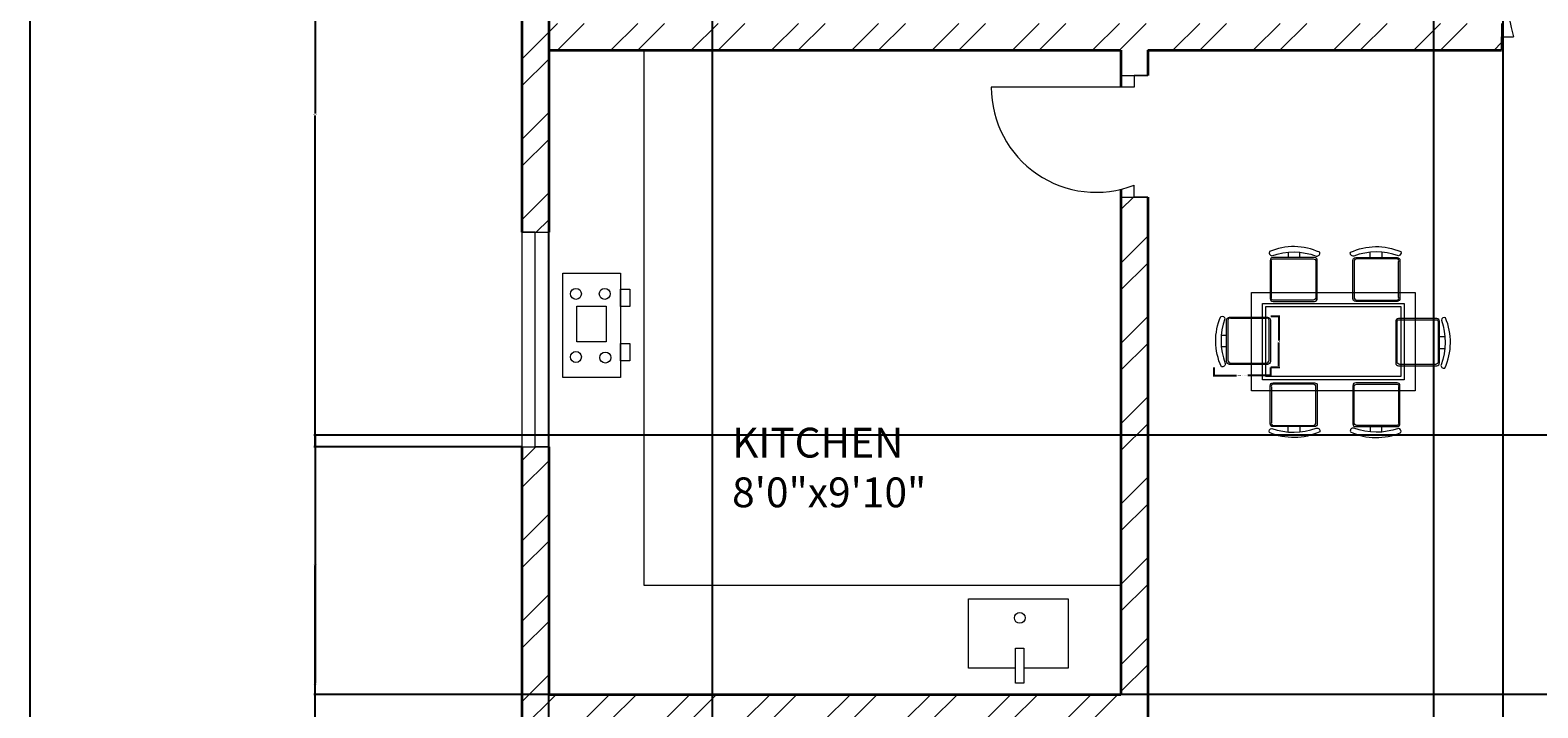
# Model space of a CAD drawing. Units: inches. Extents: x 1965 to 2673, y 1802 to 2669.
# Tile 6 of 16: x 1965 to 2218, y 2154 to 2267. Entities that reach past the tile are written whole.
import ezdxf

# ---------------------------------------------------------------- set-up
doc = ezdxf.new("R2010")
doc.units = ezdxf.units.IN
for name, color, linetype, lineweight in [('A-ANNO-DIMS', 2, 'Continuous', 18), ('A-ANNO-TTLB', 7, 'Continuous', 25), ('A-AREA-IDEN', 7, 'Continuous', 18), ('A-DOOR', 11, 'Continuous', 18), ('A-EQPM', 8, 'Continuous', 18), ('A-FLOR-CASE', 8, 'Continuous', 18), ('A-FLOR-FIXT', 9, 'Continuous', 18), ('A-FURN', 8, 'Continuous', 13), ('A-GLAZ', 181, 'Continuous', 18), ('A-WALL', 7, 'Continuous', 35), ('A-WALL-PATT', 252, 'Continuous', 13)]:
    doc.layers.add(name, color=color, linetype=linetype, lineweight=lineweight)
doc.styles.get("Standard").update_dxf_attribs({"font": 'arial.ttf'})
doc.dimstyles.get("Standard").update_dxf_attribs({"dimtxt": 0.18, "dimasz": 0.18, "dimexe": 0.18, "dimexo": 0.0625, "dimgap": 0.09, "dimtad": 0, "dimtih": 1, "dimtoh": 1, "dimdec": 4, "dimzin": 0, "dimdsep": 46, "dimtxsty": 'Standard', "dimcen": 0.09, "dimadec": 0, "dimazin": 0, "dimtfac": 1, "dimtdec": 4, "dimtofl": 0, "dimtmove": 0, "dimatfit": 3, "dimfxl": 1, "dimtolj": 1, "dimtzin": 0, "dimarcsym": 0})

# ---------------------------------------------------------------- blocks, each defined once
blk = doc.blocks.new('WIN-36IN')
for p, q in [((2.25, 36.01), (0, 36.01)), ((0, 36.01), (4.5, 36.01)), ((0, 36.01), (0, 0.01)), ((2.25, 0.01), (2.25, 36.01)), ((4.5, 36.01), (4.5, 0.01)), ((0, 0.01), (4.5, 0.01)), ((4.5, 0.01), (2.25, 0.01))]:
    blk.add_line(p, q)
blk = doc.blocks.new('TABLE-DINING-RECT')
for points in [[(0, 16.47), (27.44, 16.47), (27.44, 0), (0, 0)], [(0, 16.47), (27.44, 16.47), (27.44, 0), (0, 0)], [(1.83, 14.64), (25.61, 14.64), (25.61, 1.83), (1.83, 1.83)], [(1.83, 14.64), (25.61, 14.64), (25.61, 1.83), (1.83, 1.83)], [(2.38, 14.09), (25.06, 14.09), (25.06, 2.38), (2.38, 2.38)], [(2.38, 14.09), (25.06, 14.09), (25.06, 2.38), (2.38, 2.38)]]:
    blk.add_lwpolyline(points, close=True)
blk = doc.blocks.new('CHAIR-DINING')
for points in [[(1.58, 0.59, -0.578392), (0.96, 0.02, -0.214524), (0.85, 8.46, -0.552014), (1.52, 8.06, 0.175809), (1.58, 0.59)], [(1.58, 0.59, -0.578392), (0.96, 0.02, -0.214524), (0.85, 8.46, -0.552014), (1.52, 8.06, 0.175809), (1.58, 0.59)], [(1.82, 7.85, -0.414214), (2.31, 8.33), (8.69, 8.33, -0.414214), (9.18, 7.85), (9.18, 0.91, -0.414214), (8.69, 0.42), (2.31, 0.42, -0.414214), (1.82, 0.91), (1.82, 7.85)], [(1.82, 7.85, -0.414214), (2.31, 8.33), (8.69, 8.33, -0.414214), (9.18, 7.85), (9.18, 0.91, -0.414214), (8.69, 0.42), (2.31, 0.42, -0.414214), (1.82, 0.91), (1.82, 7.85)], [(1.82, 3.34), (0.95, 3.34, 0.064759)], [(1.82, 3.34), (0.95, 3.34, 0.064759)]]:
    blk.add_lwpolyline(points, format="xyb")
blk.add_lwpolyline([(2.04, 7.84), (2.04, 1.12, 0.414214), (2.53, 0.64), (8.47, 0.64, 0.414214), (8.96, 1.12), (8.96, 7.84, 0.512069), (8.47, 8.11), (2.53, 8.11, 0.512069)], format="xyb", close=True)
blk.add_lwpolyline([(2.04, 7.84), (2.04, 1.12, 0.414214), (2.53, 0.64), (8.47, 0.64, 0.414214), (8.96, 1.12), (8.96, 7.84, 0.512069), (8.47, 8.11), (2.53, 8.11, 0.512069)], format="xyb", close=True)
blk.add_lwpolyline([(0.93, 5.29), (1.82, 5.29)])
blk.add_lwpolyline([(0.93, 5.29), (1.82, 5.29)])
blk = doc.blocks.new('*D21')
at = {"layer": 'A-ANNO-DIMS', "color": 0, "lineweight": -2, "transparency": 16777216}
for p, q in [((2163.18, 2210.92), (2163.18, 2209.37)), ((2163.36, 2209.55), (2166.98, 2209.55)), ((2172.51, 2209.55), (2168.89, 2209.55)), ((2172.69, 2210.92), (2172.69, 2209.37))]:
    blk.add_line(p, q, dxfattribs=at)
at = {"layer": 'A-ANNO-DIMS', "color": 0, "transparency": 16777216}
for points in [[(2163.36, 2209.58), (2163.36, 2209.52), (2163.18, 2209.55)], [(2172.51, 2209.58), (2172.51, 2209.52), (2172.69, 2209.55)]]:
    blk.add_solid(points, dxfattribs=at)
at = {"layer": 'Defpoints', "color": 0, "transparency": 16777216}
for p in [(2163.18, 2210.98), (2172.69, 2210.98), (2172.69, 2209.55)]:
    blk.add_point(p, dxfattribs=at)
at = {"layer": 'A-ANNO-DIMS', "color": 0, "transparency": 16777216, "insert": (2167.94, 2209.55), "char_height": 0.18, "attachment_point": 5}
blk.add_mtext('\\A1;CHAIR 10 TYP.', dxfattribs=at)
blk = doc.blocks.new('*D22')
at = {"layer": 'A-ANNO-DIMS', "color": 0, "lineweight": -2, "transparency": 16777216}
for p, q in [((2172.75, 2219.54), (2174.29, 2219.54)), ((2174.11, 2219.36), (2174.11, 2215.44)), ((2174.11, 2211.16), (2174.11, 2215.08)), ((2172.75, 2210.98), (2174.29, 2210.98))]:
    blk.add_line(p, q, dxfattribs=at)
at = {"layer": 'A-ANNO-DIMS', "color": 0, "transparency": 16777216}
for points in [[(2174.08, 2219.36), (2174.14, 2219.36), (2174.11, 2219.54)], [(2174.08, 2211.16), (2174.14, 2211.16), (2174.11, 2210.98)]]:
    blk.add_solid(points, dxfattribs=at)
at = {"layer": 'Defpoints', "color": 0, "transparency": 16777216}
for p in [(2172.69, 2219.54), (2174.11, 2219.54), (2172.69, 2210.98)]:
    blk.add_point(p, dxfattribs=at)
at = {"layer": 'A-ANNO-DIMS', "color": 0, "transparency": 16777216, "insert": (2174.11, 2215.26), "char_height": 0.18, "attachment_point": 5}
blk.add_mtext('\\A1;9 TYP.', dxfattribs=at)
blk = doc.blocks.new('*D35')
at = {"layer": 'A-ANNO-DIMS', "color": 0, "lineweight": -2, "transparency": 16777216}
for p, q in [((2047.03, 2197.58), (2012.19, 2197.58)), ((2012.37, 2197.4), (2012.37, 2157.95)), ((2012.37, 2118.13), (2012.37, 2157.59)), ((2047.03, 2117.95), (2012.19, 2117.95))]:
    blk.add_line(p, q, dxfattribs=at)
at = {"layer": 'A-ANNO-DIMS', "color": 0, "transparency": 16777216}
for points in [[(2012.34, 2197.4), (2012.4, 2197.4), (2012.37, 2197.58)], [(2012.34, 2118.13), (2012.4, 2118.13), (2012.37, 2117.95)]]:
    blk.add_solid(points, dxfattribs=at)
at = {"layer": 'Defpoints', "color": 0, "transparency": 16777216}
for p in [(2012.37, 2197.58), (2047.09, 2197.58), (2047.09, 2117.95)]:
    blk.add_point(p, dxfattribs=at)
at = {"layer": 'A-ANNO-DIMS', "color": 0, "transparency": 16777216, "insert": (2012.37, 2157.77), "char_height": 0.18, "attachment_point": 5}
blk.add_mtext('\\A1;79.63', dxfattribs=at)
blk = doc.blocks.new('*D36')
at = {"layer": 'A-ANNO-DIMS', "color": 0, "lineweight": -2, "transparency": 16777216}
for p, q in [((2047.03, 2309.07), (2012.19, 2309.07)), ((2012.37, 2308.89), (2012.37, 2253.51)), ((2012.37, 2197.76), (2012.37, 2253.14)), ((2047.03, 2197.58), (2012.19, 2197.58))]:
    blk.add_line(p, q, dxfattribs=at)
at = {"layer": 'A-ANNO-DIMS', "color": 0, "transparency": 16777216}
for points in [[(2012.34, 2308.89), (2012.4, 2308.89), (2012.37, 2309.07)], [(2012.34, 2197.76), (2012.4, 2197.76), (2012.37, 2197.58)]]:
    blk.add_solid(points, dxfattribs=at)
at = {"layer": 'Defpoints', "color": 0, "transparency": 16777216}
for p in [(2012.37, 2309.07), (2047.09, 2309.07), (2047.09, 2197.58)]:
    blk.add_point(p, dxfattribs=at)
at = {"layer": 'A-ANNO-DIMS', "color": 0, "transparency": 16777216, "insert": (2012.37, 2253.33), "char_height": 0.18, "attachment_point": 5}
blk.add_mtext('\\A1;111.49', dxfattribs=at)
blk = doc.blocks.new('*D39')
at = {"layer": 'A-ANNO-DIMS', "color": 0, "lineweight": -2, "transparency": 16777216}
for p, q in [((2051.59, 1936.15), (2051.59, 2600.5)), ((2051.77, 2600.32), (2064.93, 2600.32)), ((2078.87, 2600.32), (2065.72, 2600.32)), ((2079.05, 1936.15), (2079.05, 2600.5))]:
    blk.add_line(p, q, dxfattribs=at)
at = {"layer": 'A-ANNO-DIMS', "color": 0, "transparency": 16777216}
for points in [[(2051.77, 2600.35), (2051.77, 2600.29), (2051.59, 2600.32)], [(2078.87, 2600.35), (2078.87, 2600.29), (2079.05, 2600.32)]]:
    blk.add_solid(points, dxfattribs=at)
at = {"layer": 'Defpoints', "color": 0, "transparency": 16777216}
for p in [(2079.05, 2600.32), (2051.59, 1936.09), (2079.05, 1936.09)]:
    blk.add_point(p, dxfattribs=at)
at = {"layer": 'A-ANNO-DIMS', "color": 0, "transparency": 16777216, "insert": (2065.32, 2600.32), "char_height": 0.18, "attachment_point": 5}
blk.add_mtext('\\A1;27.46', dxfattribs=at)
blk = doc.blocks.new('*D40')
at = {"layer": 'A-ANNO-DIMS', "color": 0, "lineweight": -2, "transparency": 16777216}
for p, q in [((2200.09, 1936.15), (2200.09, 2600.5)), ((2200.27, 2600.32), (2205.48, 2600.32)), ((2211.59, 2600.32), (2206.38, 2600.32)), ((2211.77, 1936.15), (2211.77, 2600.5))]:
    blk.add_line(p, q, dxfattribs=at)
at = {"layer": 'A-ANNO-DIMS', "color": 0, "transparency": 16777216}
for points in [[(2200.27, 2600.35), (2200.27, 2600.29), (2200.09, 2600.32)], [(2211.59, 2600.35), (2211.59, 2600.29), (2211.77, 2600.32)]]:
    blk.add_solid(points, dxfattribs=at)
at = {"layer": 'Defpoints', "color": 0, "transparency": 16777216}
for p in [(2211.77, 2600.32), (2200.09, 1936.09), (2211.77, 1936.09)]:
    blk.add_point(p, dxfattribs=at)
at = {"layer": 'A-ANNO-DIMS', "color": 0, "transparency": 16777216, "insert": (2205.93, 2600.32), "char_height": 0.18, "attachment_point": 5}
blk.add_mtext('\\A1;11.674', dxfattribs=at)
blk = doc.blocks.new('*D47')
at = {"layer": 'A-ANNO-DIMS', "color": 0, "lineweight": -2, "transparency": 16777216}
for p, q in [((2573.53, 2199.58), (2012.19, 2199.58)), ((2012.37, 2199.4), (2012.37, 2178.02)), ((2012.37, 2156.27), (2012.37, 2177.65)), ((2573.53, 2156.09), (2012.19, 2156.09))]:
    blk.add_line(p, q, dxfattribs=at)
at = {"layer": 'A-ANNO-DIMS', "color": 0, "transparency": 16777216}
for points in [[(2012.34, 2199.4), (2012.4, 2199.4), (2012.37, 2199.58)], [(2012.34, 2156.27), (2012.4, 2156.27), (2012.37, 2156.09)]]:
    blk.add_solid(points, dxfattribs=at)
at = {"layer": 'Defpoints', "color": 0, "transparency": 16777216}
for p in [(2012.37, 2199.58), (2573.59, 2199.58), (2573.59, 2156.09)]:
    blk.add_point(p, dxfattribs=at)
at = {"layer": 'A-ANNO-DIMS', "color": 0, "transparency": 16777216, "insert": (2012.37, 2177.83), "char_height": 0.18, "attachment_point": 5}
blk.add_mtext('\\A1;43.48', dxfattribs=at)

msp = doc.modelspace()

# ---------------------------------------------------------------- hatches: boundary and pattern name
at = {"layer": 'A-WALL-PATT'}
h = msp.add_hatch(dxfattribs=at)
h.set_pattern_fill('ANSI32', color=256)
h.paths.add_polyline_path([(2051.5927, 2561.0914), (2076.7559, 2561.0914), (2076.7559, 2563.3414), (2076.7559, 2565.5914), (2047.0927, 2565.5914), (2047.0927, 2518.3824), (2051.5927, 2518.3824)])
h.paths.add_polyline_path([(2051.5927, 2458.3824), (2049.3427, 2458.3824), (2047.0927, 2458.3824), (2047.0927, 2412.5914), (2248.0927, 2412.5914), (2248.0927, 2268.5914), (2252.5927, 2268.5914), (2252.5927, 2412.5914), (2252.5927, 2421.0404), (2250.3427, 2421.0404), (2248.0927, 2421.0404), (2248.0927, 2417.0914), (2051.5927, 2417.0914)])
h.paths.add_polyline_path([(2211.4933, 2268.5914), (2104.0927, 2268.5914), (2104.0927, 2272.4654), (2101.8427, 2272.4654), (2099.5927, 2272.4654), (2099.5927, 2268.5914), (2051.5927, 2268.5914), (2051.5927, 2264.0914), (2147.5927, 2264.0914), (2147.5927, 2259.8893), (2152.0927, 2259.8893), (2152.0927, 2264.0914), (2211.4933, 2264.0914), (2211.4933, 2266.3414)])
h.paths.add_polyline_path([(2104.0927, 2376.0914), (2099.5927, 2376.0914), (2047.0927, 2376.0914), (2047.0927, 2333.0682), (2051.5927, 2333.0682), (2051.5927, 2371.5914), (2099.5927, 2371.5914), (2099.5927, 2293.6123), (2104.0927, 2293.6123)], flags=17)
h.paths.add_polyline_path([(2051.5927, 2309.0682), (2047.0927, 2309.0682), (2047.0927, 2233.5821), (2051.5927, 2233.5821)])
h.paths.add_polyline_path([(2104.0927, 2412.5914), (2099.5927, 2412.5914), (2099.5927, 2376.0914), (2104.0927, 2376.0914)], flags=17)
h.paths.add_polyline_path([(2290.1254, 2268.5914), (2242.4924, 2268.5914), (2242.4924, 2264.0914), (2290.1254, 2264.0914), (2290.1254, 2266.3414)])
h.paths.add_polyline_path([(2284.653, 2264.0914), (2280.153, 2264.0914), (2280.153, 2161.6826), (2284.653, 2161.6826)])
h.paths.add_polyline_path([(2578.0927, 2329.4656), (2573.5927, 2329.4656), (2573.5927, 2268.5914), (2525.5927, 2268.5914), (2525.5927, 2271.9222), (2523.3427, 2271.9222), (2521.0927, 2271.9222), (2521.0927, 2268.5914), (2324.2835, 2268.5914), (2324.2835, 2264.0914), (2329.0927, 2264.0914), (2329.0927, 2259.4977), (2333.5927, 2259.4977), (2333.5927, 2264.0914), (2473.0927, 2264.0914), (2473.0927, 2259.9371), (2477.5927, 2259.9371), (2477.5927, 2264.0914), (2573.5927, 2264.0914), (2573.5927, 2235.5751), (2578.0927, 2235.5751)])
h.paths.add_polyline_path([(2377.0927, 2412.5914), (2578.0927, 2412.5914), (2578.0927, 2444.2286), (2575.8427, 2444.2286), (2573.5927, 2444.2286), (2573.5927, 2417.0914), (2429.5927, 2417.0914), (2377.0927, 2417.0914), (2377.0927, 2421.7443), (2372.5927, 2421.7443), (2372.5927, 2268.5914), (2377.0927, 2268.5914)])
h.paths.add_polyline_path([(2525.5927, 2371.5914), (2573.5927, 2371.5914), (2573.5927, 2353.4656), (2578.0927, 2353.4656), (2578.0927, 2376.0914), (2525.5927, 2376.0914), (2521.0927, 2376.0914), (2521.0927, 2290.6472), (2525.5927, 2290.6472)], flags=17)
h.paths.add_polyline_path([(2477.5927, 2236.4106), (2475.3427, 2236.4106), (2473.0927, 2236.4106), (2473.0927, 2084.5914), (2465.3309, 2084.5914), (2465.3309, 2080.0914), (2481.6764, 2080.0914), (2481.6764, 2082.3414), (2481.6764, 2084.5914), (2477.5927, 2084.5914), (2477.5927, 2151.5914), (2573.5927, 2151.5914), (2573.5927, 2130.2907), (2578.0927, 2130.2907), (2578.0927, 2199.5751), (2575.8427, 2199.5751), (2573.5927, 2199.5751), (2573.5927, 2156.0914), (2477.5927, 2156.0914)])
h.paths.add_polyline_path([(2573.5927, 2084.5914), (2505.5513, 2084.5914), (2505.5513, 2080.0914), (2573.5927, 2080.0914)], flags=17)
h.paths.add_polyline_path([(2578.0927, 2106.2907), (2575.8427, 2106.2907), (2573.5927, 2106.2907), (2573.5927, 2050.8986), (2578.0927, 2050.8986)])
h.paths.add_polyline_path([(2578.0927, 1990.8986), (2575.8427, 1990.8986), (2573.5927, 1990.8986), (2573.5927, 1936.0914), (2522.132, 1936.0914), (2522.132, 1931.5914), (2578.0927, 1931.5914)])
h.paths.add_polyline_path([(2462.132, 1936.0914), (2429.5927, 1936.0914), (2429.5927, 2080.0914), (2432.623, 2080.0914), (2432.623, 2082.3414), (2432.623, 2084.5914), (2429.5927, 2084.5914), (2429.5927, 2120.5914), (2333.5927, 2120.5914), (2333.5927, 2229.3125), (2331.3427, 2229.3125), (2329.0927, 2229.3125), (2329.0927, 2116.0914), (2425.0927, 2116.0914), (2425.0927, 1936.0914), (2346.4058, 1936.0914), (2346.4058, 1931.5914), (2462.132, 1931.5914), (2462.132, 1933.8414)])
h.paths.add_polyline_path([(2211.767, 1933.8414), (2211.767, 1936.0914), (2200.0927, 1936.0914), (2200.0927, 2080.0914), (2200.0927, 2116.0914), (2284.653, 2116.0914), (2284.653, 2130.591), (2282.403, 2130.591), (2280.153, 2130.591), (2280.153, 2120.5914), (2200.0927, 2120.5914), (2195.5927, 2120.5914), (2195.5927, 2080.0914), (2195.5927, 1936.0914), (2139.0533, 1936.0914), (2139.0533, 1931.5914), (2211.767, 1931.5914)])
h.paths.add_polyline_path([(2282.2502, 1933.8414), (2282.2502, 1936.0914), (2259.767, 1936.0914), (2259.767, 1931.5914), (2282.2502, 1931.5914)], flags=17)
h.paths.add_polyline_path([(2051.5927, 1987.096), (2049.3427, 1987.096), (2047.0927, 1987.096), (2047.0927, 1931.5914), (2079.0533, 1931.5914), (2079.0533, 1933.8414), (2079.0533, 1936.0914), (2051.5927, 1936.0914)])
h.paths.add_polyline_path([(2051.5927, 2197.5821), (2049.3427, 2197.5821), (2047.0927, 2197.5821), (2047.0927, 2141.952), (2051.5927, 2141.952), (2051.5927, 2151.5914), (2147.5927, 2151.5914), (2147.5927, 2084.5914), (2144.3652, 2084.5914), (2144.3652, 2080.0914), (2155.9662, 2080.0914), (2155.9662, 2082.3414), (2155.9662, 2084.5914), (2152.0927, 2084.5914), (2152.0927, 2239.4921), (2149.8427, 2239.4921), (2147.5927, 2239.4921), (2147.5927, 2156.0914), (2051.5927, 2156.0914)])
h.paths.add_polyline_path([(2051.5927, 2080.0914), (2123.8575, 2080.0914), (2123.8575, 2082.3414), (2123.8575, 2084.5914), (2051.5927, 2084.5914), (2051.5927, 2117.952), (2047.0927, 2117.952), (2047.0927, 2047.096), (2051.5927, 2047.096)])
h = msp.add_hatch(dxfattribs=at)
h.set_pattern_fill('ANSI32', color=256)
h.paths.add_polyline_path([(2210.2316, 2563.3414), (2210.2316, 2565.5914), (2136.7559, 2565.5914), (2136.7559, 2561.0914), (2195.5927, 2561.0914), (2195.5927, 2485.8604), (2200.0927, 2485.8604), (2200.0927, 2561.0914), (2210.2316, 2561.0914)])
h.paths.add_polyline_path([(2285.9734, 2565.5914), (2234.2316, 2565.5914), (2234.2316, 2561.0914), (2248.0927, 2561.0914), (2248.0927, 2462.0914), (2200.0927, 2462.0914), (2200.0927, 2465.2357), (2197.8427, 2465.2357), (2195.5927, 2465.2357), (2195.5927, 2457.5914), (2248.0927, 2457.5914), (2248.0927, 2452.628), (2252.5927, 2452.628), (2252.5927, 2457.5914), (2257.5156, 2457.5914), (2257.5156, 2459.8414), (2257.5156, 2462.0914), (2252.5927, 2462.0914), (2252.5927, 2561.0914), (2285.9734, 2561.0914)])
h.paths.add_polyline_path([(2213.1374, 1872.8885), (2461.061, 1872.8885), (2461.061, 1909.9813), (2213.1374, 1909.9813)], flags=9)
h.paths.add_polyline_path([(2328.4056, 1942.3944), (2340.6089, 1942.3944), (2340.6089, 1952.6979), (2328.4056, 1952.6979)], flags=9)
h.paths.add_polyline_path([(2353.5759, 2030.9808), (2376.6455, 2030.9808), (2376.6455, 2041.2844), (2353.5759, 2041.2844)], flags=9)
h.paths.add_polyline_path([(2289.989, 2074.1041), (2326.916, 2074.1041), (2326.916, 2092.7615), (2289.989, 2092.7615)], flags=9)
h.paths.add_polyline_path([(2497.9, 2052.8638), (2548.3741, 2052.8638), (2548.3741, 2071.5212), (2497.9, 2071.5212)], flags=9)
h.paths.add_polyline_path([(2486.59, 2116.4883), (2515.7475, 2116.4883), (2515.7475, 2135.1456), (2486.59, 2135.1456)], flags=9)
h.paths.add_polyline_path([(2497.3007, 2181.2877), (2530.459, 2181.2877), (2530.459, 2199.945), (2497.3007, 2199.945)], flags=9)
h.paths.add_polyline_path([(2288.237, 2190.3228), (2324.1238, 2190.3228), (2324.1238, 2208.9802), (2288.237, 2208.9802)], flags=9)
h.paths.add_polyline_path([(2350.806, 2127.8307), (2387.733, 2127.8307), (2387.733, 2146.488), (2350.806, 2146.488)], flags=9)
h.paths.add_polyline_path([(2530.3237, 2315.2679), (2559.5563, 2315.2679), (2559.5563, 2333.9252), (2530.3237, 2333.9252)], flags=9)
h.paths.add_polyline_path([(2418.419, 2383.4707), (2468.2894, 2383.4707), (2468.2894, 2402.1281), (2418.419, 2402.1281)], flags=9)
h.paths.add_polyline_path([(2327.4503, 2399.0281), (2364.3773, 2399.0281), (2364.3773, 2417.6854), (2327.4503, 2417.6854)], flags=9)
h.paths.add_polyline_path([(2147.9722, 2271.4601), (2197.8426, 2271.4601), (2197.8426, 2290.1174), (2147.9722, 2290.1174)], flags=9)
h.paths.add_polyline_path([(2474.3875, 2421.594), (2524.8616, 2421.594), (2524.8616, 2440.2514), (2474.3875, 2440.2514)], flags=9)
h.paths.add_polyline_path([(2063.9863, 2052.9059), (2114.4604, 2052.9059), (2114.4604, 2071.5632), (2063.9863, 2071.5632)], flags=9)
h.paths.add_polyline_path([(2200.3335, 2133.7067), (2237.2605, 2133.7067), (2237.2605, 2152.364), (2200.3335, 2152.364)], flags=9)
h.paths.add_polyline_path([(2080.5973, 2184.636), (2113.8681, 2184.636), (2113.8681, 2203.2933), (2080.5973, 2203.2933)], flags=9)
h.paths.add_polyline_path([(2102.4918, 2116.4497), (2131.6494, 2116.4497), (2131.6494, 2135.107), (2102.4918, 2135.107)], flags=9)
h.paths.add_polyline_path([(2056.2753, 2308.5576), (2085.5079, 2308.5576), (2085.5079, 2327.2149), (2056.2753, 2327.2149)], flags=9)
h.paths.add_polyline_path([(2385.619, 2500.9729), (2414.8516, 2500.9729), (2414.8516, 2519.6303), (2385.619, 2519.6303)], flags=9)
h.paths.add_polyline_path([(2286.6643, 2508.6826), (2320.0715, 2508.6826), (2320.0715, 2527.34), (2286.6643, 2527.34)], flags=9)
h.paths.add_polyline_path([(2206.5604, 2500.7243), (2235.793, 2500.7243), (2235.793, 2519.3817), (2206.5604, 2519.3817)], flags=25)
h.paths.add_polyline_path([(2062.6644, 2424.4027), (2112.5348, 2424.4027), (2112.5348, 2443.0601), (2062.6644, 2443.0601)], flags=9)
h = msp.add_hatch(dxfattribs=at)
h.set_pattern_fill('ANSI32', color=256)
h.paths.add_polyline_path([(2429.5927, 2468.6101), (2427.3427, 2468.6101), (2425.0927, 2468.6101), (2425.0927, 2462.0914), (2377.0927, 2462.0914), (2377.0927, 2561.0914), (2390.4173, 2561.0914), (2390.4173, 2565.5914), (2321.9734, 2565.5914), (2321.9734, 2561.0914), (2372.5927, 2561.0914), (2372.5927, 2462.0914), (2281.6605, 2462.0914), (2281.6605, 2457.5914), (2372.5927, 2457.5914), (2372.5927, 2451.3316), (2377.0927, 2451.3316), (2377.0927, 2457.5914), (2429.5927, 2457.5914)])
h.paths.add_polyline_path([(2480.8929, 2565.5914), (2414.4173, 2565.5914), (2414.4173, 2561.0914), (2425.0927, 2561.0914), (2425.0927, 2489.9153), (2429.5927, 2489.9153), (2429.5927, 2561.0914), (2480.8929, 2561.0914), (2480.8929, 2563.3414)])
h.paths.add_polyline_path([(2213.1374, 1872.8885), (2461.061, 1872.8885), (2461.061, 1909.9813), (2213.1374, 1909.9813)], flags=9)
h.paths.add_polyline_path([(2328.4056, 1942.3944), (2340.6089, 1942.3944), (2340.6089, 1952.6979), (2328.4056, 1952.6979)], flags=9)
h.paths.add_polyline_path([(2353.5759, 2030.9808), (2376.6455, 2030.9808), (2376.6455, 2041.2844), (2353.5759, 2041.2844)], flags=9)
h.paths.add_polyline_path([(2289.989, 2074.1041), (2326.916, 2074.1041), (2326.916, 2092.7615), (2289.989, 2092.7615)], flags=9)
h.paths.add_polyline_path([(2497.9, 2052.8638), (2548.3741, 2052.8638), (2548.3741, 2071.5212), (2497.9, 2071.5212)], flags=9)
h.paths.add_polyline_path([(2486.59, 2116.4883), (2515.7475, 2116.4883), (2515.7475, 2135.1456), (2486.59, 2135.1456)], flags=9)
h.paths.add_polyline_path([(2497.3007, 2181.2877), (2530.459, 2181.2877), (2530.459, 2199.945), (2497.3007, 2199.945)], flags=9)
h.paths.add_polyline_path([(2288.237, 2190.3228), (2324.1238, 2190.3228), (2324.1238, 2208.9802), (2288.237, 2208.9802)], flags=9)
h.paths.add_polyline_path([(2350.806, 2127.8307), (2387.733, 2127.8307), (2387.733, 2146.488), (2350.806, 2146.488)], flags=9)
h.paths.add_polyline_path([(2530.3237, 2315.2679), (2559.5563, 2315.2679), (2559.5563, 2333.9252), (2530.3237, 2333.9252)], flags=9)
h.paths.add_polyline_path([(2418.419, 2383.4707), (2468.2894, 2383.4707), (2468.2894, 2402.1281), (2418.419, 2402.1281)], flags=9)
h.paths.add_polyline_path([(2327.4503, 2399.0281), (2364.3773, 2399.0281), (2364.3773, 2417.6854), (2327.4503, 2417.6854)], flags=9)
h.paths.add_polyline_path([(2147.9722, 2271.4601), (2197.8426, 2271.4601), (2197.8426, 2290.1174), (2147.9722, 2290.1174)], flags=9)
h.paths.add_polyline_path([(2474.3875, 2421.594), (2524.8616, 2421.594), (2524.8616, 2440.2514), (2474.3875, 2440.2514)], flags=9)
h.paths.add_polyline_path([(2063.9863, 2052.9059), (2114.4604, 2052.9059), (2114.4604, 2071.5632), (2063.9863, 2071.5632)], flags=9)
h.paths.add_polyline_path([(2200.3335, 2133.7067), (2237.2605, 2133.7067), (2237.2605, 2152.364), (2200.3335, 2152.364)], flags=9)
h.paths.add_polyline_path([(2080.5973, 2184.636), (2113.8681, 2184.636), (2113.8681, 2203.2933), (2080.5973, 2203.2933)], flags=9)
h.paths.add_polyline_path([(2102.4918, 2116.4497), (2131.6494, 2116.4497), (2131.6494, 2135.107), (2102.4918, 2135.107)], flags=9)
h.paths.add_polyline_path([(2056.2753, 2308.5576), (2085.5079, 2308.5576), (2085.5079, 2327.2149), (2056.2753, 2327.2149)], flags=9)
h.paths.add_polyline_path([(2385.619, 2500.9729), (2414.8516, 2500.9729), (2414.8516, 2519.6303), (2385.619, 2519.6303)], flags=25)
h.paths.add_polyline_path([(2286.6643, 2508.6826), (2320.0715, 2508.6826), (2320.0715, 2527.34), (2286.6643, 2527.34)], flags=25)
h.paths.add_polyline_path([(2206.5604, 2500.7243), (2235.793, 2500.7243), (2235.793, 2519.3817), (2206.5604, 2519.3817)], flags=9)
h.paths.add_polyline_path([(2062.6644, 2424.4027), (2112.5348, 2424.4027), (2112.5348, 2443.0601), (2062.6644, 2443.0601)], flags=9)

# ---------------------------------------------------------------- linework, layer by layer
at = {"layer": 'A-ANNO-TTLB'}
msp.add_lwpolyline([(1964.5703, 2669.282), (2673.2605, 2669.282), (2673.2605, 1802.0221), (1964.5703, 1802.0221)], close=True, dxfattribs=at)
at = {"layer": 'A-DOOR'}
for p, q in [((2211.4933, 2268.5914), (2211.4933, 2264.0914)), ((2211.4933, 2264.0914), (2211.4933, 2266.3414)), ((2211.4933, 2266.3414), (2211.4933, 2266.3414)), ((2211.4933, 2266.3414), (2213.4933, 2266.3414)), ((2147.5927, 2259.8893), (2152.0927, 2259.8893)), ((2152.0927, 2259.8893), (2149.8427, 2259.8893)), ((2149.8427, 2259.8893), (2149.8427, 2257.8893)), ((2149.8427, 2257.8893), (2125.8427, 2257.8893)), ((2147.5927, 2239.4921), (2152.0927, 2239.4921)), ((2149.8427, 2239.4921), (2149.8427, 2241.4921)), ((2152.0927, 2239.4921), (2149.8427, 2239.4921))]:
    msp.add_line(p, q, dxfattribs=at)
for centre, radius, start, end in [((2240.4924, 2274.217), 28.1243, 90, 196.261997), ((2143.4441, 2257.8893), 17.6014, 180, 291.317095)]:
    msp.add_arc(centre, radius, start, end, dxfattribs=at)
at = {"layer": 'A-EQPM'}
for points in [[(2053.9419, 2226.7496), (2063.6145, 2226.7496), (2063.6145, 2209.2028), (2053.9419, 2209.2028)], [(2063.6145, 2224.0351), (2065.1828, 2224.0351), (2065.1828, 2221.155), (2063.6145, 2221.155)], [(2056.2917, 2221.2066), (2061.2334, 2221.2066), (2061.2334, 2215.1825), (2056.2917, 2215.1825)], [(2063.6145, 2214.9304), (2065.1828, 2214.9304), (2065.1828, 2212.0503), (2063.6145, 2212.0503)]]:
    msp.add_lwpolyline(points, close=True, dxfattribs=at)
for centre in [(2056.151, 2223.2548), (2060.9924, 2223.2548), (2056.151, 2212.6724), (2061.0928, 2212.572)]:
    msp.add_circle(centre, 0.9237, dxfattribs=at)
at = {"layer": 'A-FLOR-CASE'}
for p, q in [((2067.5569, 2264.0914), (2067.5569, 2174.4181)), ((2067.5569, 2174.4181), (2147.5927, 2174.4181))]:
    msp.add_line(p, q, dxfattribs=at)
at = {"layer": 'A-FLOR-FIXT'}
msp.add_lwpolyline([(2129.9348, 2160.4719), (2122.0193, 2160.4719), (2122.0193, 2172.096), (2138.7623, 2172.096), (2138.7623, 2160.4719), (2131.3354, 2160.4719)], dxfattribs=at)
msp.add_lwpolyline([(2129.9348, 2163.8257), (2131.3354, 2163.8257), (2131.3354, 2157.9973), (2129.9348, 2157.9973)], close=True, dxfattribs=at)
msp.add_circle((2130.6351, 2168.9245), 0.9076, dxfattribs=at)
at = {"layer": 'A-FURN'}
for points in [[(2172.9118, 2229.6509, -0.17580919), (2180.3872, 2229.5943, 0.57839206), (2180.9535, 2230.217, 0.21452438), (2172.5153, 2230.3302, 0.55201397), (2172.9118, 2229.6509, -0.06507904)], [(2172.9118, 2229.6506, -0.17580919), (2180.3872, 2229.594, 0.57839206), (2180.9535, 2230.2167, 0.21452438), (2172.5154, 2230.3299, 0.55201397), (2172.9118, 2229.6506, -0.06507904)], [(2180.0701, 2229.3508), (2173.1301, 2229.3508, 0.41421356), (2172.6446, 2228.8653), (2172.6446, 2222.4842, 0.41421356), (2173.1301, 2221.9987), (2180.0701, 2221.9987, 0.41421356), (2180.5556, 2222.4842), (2180.5556, 2228.8653, 0.41421356), (2180.0701, 2229.3508)], [(2180.0701, 2229.3506), (2173.1301, 2229.3506, 0.41421356), (2172.6446, 2228.865), (2172.6446, 2222.4839, 0.41421356), (2173.1301, 2221.9984), (2180.0701, 2221.9984, 0.41421356), (2180.5556, 2222.4839), (2180.5556, 2228.865, 0.41421356), (2180.0701, 2229.3506)], [(2177.6324, 2229.3508), (2177.6324, 2230.2285, -0.06475861)], [(2177.6324, 2229.3506), (2177.6324, 2230.2282, -0.06475861)], [(2186.6806, 2229.5943, -0.57839206), (2186.1142, 2230.217, -0.21452438), (2194.5524, 2230.3302, -0.55201397), (2194.156, 2229.6509, 0.1758092), (2186.6806, 2229.5943)], [(2186.6806, 2229.594, -0.57839206), (2186.1143, 2230.2167, -0.21452438), (2194.5524, 2230.3299, -0.55201397), (2194.156, 2229.6506, 0.1758092), (2186.6806, 2229.594)], [(2193.9377, 2229.3508, -0.41421356), (2194.4232, 2228.8653), (2194.4232, 2222.4842, -0.41421356), (2193.9377, 2221.9987), (2186.9977, 2221.9987, -0.41421356), (2186.5122, 2222.4842), (2186.5122, 2228.8653, -0.41421356), (2186.9977, 2229.3508), (2193.9377, 2229.3508)], [(2193.9377, 2229.3506, -0.41421356), (2194.4232, 2228.865), (2194.4232, 2222.4839, -0.41421356), (2193.9377, 2221.9984), (2186.9977, 2221.9984, -0.41421356), (2186.5122, 2222.4839), (2186.5122, 2228.865, -0.41421356), (2186.9977, 2229.3506), (2193.9377, 2229.3506)], [(2189.4354, 2229.3508), (2189.4354, 2230.2285, 0.06475861)], [(2189.4354, 2229.3506), (2189.4354, 2230.2282, 0.06475861)], [(2201.0719, 2218.6182, 0.41421356), (2200.5864, 2219.1038), (2194.2052, 2219.1038, 0.41421356), (2193.7197, 2218.6182), (2193.7197, 2211.6783, 0.41421356), (2194.2052, 2211.1928), (2200.5864, 2211.1928, 0.41421356), (2201.0719, 2211.6783), (2201.0719, 2218.6182)], [(2201.0719, 2218.618, 0.41421356), (2200.5864, 2219.1035), (2194.2052, 2219.1035, 0.41421356), (2193.7197, 2218.618), (2193.7197, 2211.678, 0.41421356), (2194.2052, 2211.1925), (2200.5864, 2211.1925, 0.41421356), (2201.0719, 2211.678), (2201.0719, 2218.618)], [(2201.3719, 2218.8366, -0.17580919), (2201.3153, 2211.3612, 0.57839206), (2201.938, 2210.7948, 0.21452438), (2202.0513, 2219.233, 0.55201397), (2201.3719, 2218.8366, -0.06507904)], [(2201.3719, 2218.8363, -0.17580919), (2201.3153, 2211.3609, 0.57839206), (2201.9381, 2210.7945, 0.21452438), (2202.0513, 2219.2327, 0.55201397), (2201.3719, 2218.8363, -0.06507904)], [(2201.0719, 2214.116), (2201.9496, 2214.116, -0.06475861)], [(2201.0719, 2214.1157), (2201.9496, 2214.1157, -0.06475861)], [(2180.0701, 2200.9851), (2173.1301, 2200.9851, -0.41421356), (2172.6446, 2201.4706), (2172.6446, 2207.8518, -0.41421356), (2173.1301, 2208.3373), (2180.0701, 2208.3373, -0.41421356), (2180.5556, 2207.8518), (2180.5556, 2201.4706, -0.41421356), (2180.0701, 2200.9851)], [(2180.0701, 2200.9848), (2173.1301, 2200.9848, -0.41421356), (2172.6446, 2201.4703), (2172.6446, 2207.8515, -0.41421356), (2173.1301, 2208.337), (2180.0701, 2208.337, -0.41421356), (2180.5556, 2207.8515), (2180.5556, 2201.4703, -0.41421356), (2180.0701, 2200.9848)], [(2193.9377, 2200.9851, 0.41421356), (2194.4232, 2201.4706), (2194.4232, 2207.8518, 0.41421356), (2193.9377, 2208.3373), (2186.9977, 2208.3373, 0.41421356), (2186.5122, 2207.8518), (2186.5122, 2201.4706, 0.41421356), (2186.9977, 2200.9851), (2193.9377, 2200.9851)], [(2193.9377, 2200.9848, 0.41421356), (2194.4232, 2201.4703), (2194.4232, 2207.8515, 0.41421356), (2193.9377, 2208.337), (2186.9977, 2208.337, 0.41421356), (2186.5122, 2207.8515), (2186.5122, 2201.4703, 0.41421356), (2186.9977, 2200.9848), (2193.9377, 2200.9848)], [(2180.3872, 2200.7417, -0.57839206), (2180.9535, 2200.119, -0.21452438), (2172.5153, 2200.0057, -0.55201397), (2172.9118, 2200.6851, 0.17580929), (2180.3872, 2200.7417)], [(2180.3872, 2200.7414, -0.57839206), (2180.9535, 2200.1187, -0.21452438), (2172.5154, 2200.0055, -0.55201397), (2172.9118, 2200.6848, 0.17580929), (2180.3872, 2200.7414)], [(2177.6324, 2200.9851), (2177.6324, 2200.1074, 0.06475861)], [(2177.6324, 2200.9848), (2177.6324, 2200.1071, 0.06475861)], [(2194.156, 2200.6851, -0.17580928), (2186.6806, 2200.7417, 0.57839206), (2186.1142, 2200.119, 0.21452438), (2194.5524, 2200.0057, 0.55201397), (2194.156, 2200.6851, -0.06507904)], [(2194.156, 2200.6848, -0.17580928), (2186.6806, 2200.7414, 0.57839206), (2186.1143, 2200.1187, 0.21452438), (2194.5524, 2200.0055, 0.55201397), (2194.156, 2200.6848, -0.06507904)], [(2189.4354, 2200.9851), (2189.4354, 2200.1074, -0.06475861)], [(2189.4354, 2200.9848), (2189.4354, 2200.1071, -0.06475861)]]:
    msp.add_lwpolyline(points, format="xyb", dxfattribs=at)
for points in [[(2173.1331, 2229.1321), (2179.8513, 2229.1321, -0.41421356), (2180.3368, 2228.6466), (2180.3368, 2222.7029, -0.41421356), (2179.8513, 2222.2174), (2173.1331, 2222.2174, -0.51206948), (2172.8633, 2222.7029), (2172.8633, 2228.6466, -0.51206948)], [(2173.1331, 2229.1318), (2179.8513, 2229.1318, -0.41421356), (2180.3369, 2228.6463), (2180.3369, 2222.7026, -0.41421356), (2179.8513, 2222.2171), (2173.1331, 2222.2171, -0.51206948), (2172.8633, 2222.7026), (2172.8633, 2228.6463, -0.51206948)], [(2193.9347, 2229.1321), (2187.2164, 2229.1321, 0.41421356), (2186.7309, 2228.6466), (2186.7309, 2222.7029, 0.41421356), (2187.2164, 2222.2174), (2193.9347, 2222.2174, 0.51206948), (2194.2044, 2222.7029), (2194.2044, 2228.6466, 0.51206948)], [(2193.9347, 2229.1318), (2187.2165, 2229.1318, 0.41421356), (2186.7309, 2228.6463), (2186.7309, 2222.7026, 0.41421356), (2187.2165, 2222.2171), (2193.9347, 2222.2171, 0.51206948), (2194.2045, 2222.7026), (2194.2045, 2228.6463, 0.51206948)], [(2200.8532, 2218.6153), (2200.8532, 2211.897, -0.41421356), (2200.3676, 2211.4115), (2194.424, 2211.4115, -0.41421356), (2193.9384, 2211.897), (2193.9384, 2218.6153, -0.51206948), (2194.424, 2218.885), (2200.3676, 2218.885, -0.51206948)], [(2200.8532, 2218.615), (2200.8532, 2211.8967, -0.41421356), (2200.3677, 2211.4112), (2194.424, 2211.4112, -0.41421356), (2193.9385, 2211.8967), (2193.9385, 2218.615, -0.51206948), (2194.424, 2218.8847), (2200.3677, 2218.8847, -0.51206948)], [(2173.1331, 2201.2038), (2179.8513, 2201.2038, 0.41421356), (2180.3368, 2201.6894), (2180.3368, 2207.633, 0.41421356), (2179.8513, 2208.1186), (2173.1331, 2208.1186, 0.51206948), (2172.8633, 2207.633), (2172.8633, 2201.6894, 0.51206948)], [(2173.1331, 2201.2035), (2179.8513, 2201.2035, 0.41421356), (2180.3369, 2201.6891), (2180.3369, 2207.6327, 0.41421356), (2179.8513, 2208.1183), (2173.1331, 2208.1183, 0.51206948), (2172.8633, 2207.6327), (2172.8633, 2201.6891, 0.51206948)], [(2193.9347, 2201.2038), (2187.2164, 2201.2038, -0.41421356), (2186.7309, 2201.6894), (2186.7309, 2207.633, -0.41421356), (2187.2164, 2208.1186), (2193.9347, 2208.1186, -0.51206948), (2194.2044, 2207.633), (2194.2044, 2201.6894, -0.51206948)], [(2193.9347, 2201.2035), (2187.2165, 2201.2035, -0.41421356), (2186.7309, 2201.6891), (2186.7309, 2207.6327, -0.41421356), (2187.2165, 2208.1183), (2193.9347, 2208.1183, -0.51206948), (2194.2045, 2207.6327), (2194.2045, 2201.6891, -0.51206948)]]:
    msp.add_lwpolyline(points, format="xyb", close=True, dxfattribs=at)
for points in [[(2175.6898, 2230.2445), (2175.6898, 2229.3508)], [(2175.6898, 2230.2442), (2175.6898, 2229.3506)], [(2191.378, 2230.2445), (2191.378, 2229.3508)], [(2191.378, 2230.2442), (2191.378, 2229.3506)], [(2201.9655, 2216.0586), (2201.0719, 2216.0586)], [(2201.9656, 2216.0583), (2201.0719, 2216.0583)], [(2175.6898, 2200.0915), (2175.6898, 2200.9851)], [(2175.6898, 2200.0912), (2175.6898, 2200.9848)], [(2191.378, 2200.0915), (2191.378, 2200.9851)], [(2191.378, 2200.0912), (2191.378, 2200.9848)]]:
    msp.add_lwpolyline(points, dxfattribs=at)
at = {"layer": 'A-WALL'}
for p, q in [((2047.0927, 2309.0682), (2047.0927, 2233.5821)), ((2051.5927, 2309.0682), (2051.5927, 2233.5821)), ((2051.5927, 2264.0914), (2147.5927, 2264.0914)), ((2147.5927, 2264.0914), (2147.5927, 2257.8893)), ((2152.0927, 2264.0914), (2152.0927, 2259.8893)), ((2152.0927, 2264.0914), (2211.4933, 2264.0914)), ((2147.5927, 2240.7838), (2147.5927, 2156.0914)), ((2152.0927, 2239.4921), (2152.0927, 2084.5914)), ((2047.0927, 2197.5821), (2047.0927, 2141.952)), ((2051.5927, 2197.5821), (2051.5927, 2156.0914)), ((2051.5927, 2156.0914), (2147.5927, 2156.0914)), ((2051.5927, 2156.0914), (2147.5927, 2156.0914))]:
    msp.add_line(p, q, dxfattribs=at)

# ---------------------------------------------------------------- block references
at = {"layer": 'A-FURN'}
for name, p in [('TABLE-DINING-RECT', (2169.52, 2207.02)), ('CHAIR-DINING', (2163.51, 2211.01))]:
    msp.add_blockref(name, p, dxfattribs=at)
at = {"layer": 'A-GLAZ'}
msp.add_blockref('WIN-36IN', (2047.09, 2197.5771), dxfattribs=at)

# ---------------------------------------------------------------- texts
at = {"layer": 'A-AREA-IDEN', "insert": (2082.3589, 2200.8052), "char_height": 5, "attachment_point": 1}
msp.add_mtext_dynamic_manual_height_columns('KITCHEN\\P8\'0"x9\'10"', width=251.233811, gutter_width=12.5, heights=[0], dxfattribs=at)

# ---------------------------------------------------------------- dimensions: what is measured, and where the dimension line sits
at = {"layer": 'A-ANNO-DIMS'}
for base, p1, p2, override, picture, middle in [((2079.0533, 2600.3164), (2051.5927, 1936.0914), (2079.0533, 1936.0914), {"dimdec": 2, "dimlfac": 1, "dimrnd": 0, "dimzin": 0, "dimdsep": 46, "dimlunit": 2}, '*D39', (2065.323, 2600.3164)), ((2211.767, 2600.3164), (2200.0927, 1936.0914), (2211.767, 1936.0914), {"dimdec": 3, "dimlfac": 1, "dimrnd": 0, "dimzin": 0, "dimdsep": 46, "dimlunit": 2}, '*D40', (2205.9299, 2600.3164))]:
    dim = msp.add_linear_dim(base=base, p1=p1, p2=p2, dimstyle='Standard', override=override, dxfattribs=at)
    dim.commit()
    dim.dimension.update_dxf_attribs({"geometry": picture, "text_midpoint": middle})
for base, p1, p2, picture, middle in [((2012.3677, 2309.0682), (2047.0927, 2197.5821), (2047.0927, 2309.0682), '*D36', (2012.3677, 2253.3252)), ((2012.3677, 2199.5751), (2573.5927, 2156.0914), (2573.5927, 2199.5751), '*D47', (2012.3677, 2177.8332)), ((2012.3677, 2197.5821), (2047.0927, 2117.952), (2047.0927, 2197.5821), '*D35', (2012.3677, 2157.7671))]:
    dim = msp.add_linear_dim(base=base, p1=p1, p2=p2, angle=90, dimstyle='Standard', override={"dimdec": 2, "dimlfac": 1, "dimrnd": 0, "dimzin": 0, "dimdsep": 46, "dimlunit": 2}, dxfattribs=at)
    dim.commit()
    dim.dimension.update_dxf_attribs({"geometry": picture, "text_midpoint": middle})
dim = msp.add_linear_dim(base=(2174.112, 2219.5445), p1=(2172.6867, 2210.9791), p2=(2172.6867, 2219.5445), angle=90, text='<> TYP.', dimstyle='Standard', override={"dimdec": 0, "dimlfac": 1, "dimrnd": 0, "dimzin": 0, "dimdsep": 46, "dimlunit": 2}, dxfattribs=at)
dim.commit()
dim.dimension.update_dxf_attribs({"geometry": '*D22', "text_midpoint": (2174.112, 2215.2618)})
dim = msp.add_linear_dim(base=(2172.6867, 2209.5537), p1=(2163.1843, 2210.9791), p2=(2172.6867, 2210.9791), text='CHAIR <> TYP.', dimstyle='Standard', override={"dimdec": 0, "dimlfac": 1, "dimrnd": 0, "dimzin": 0, "dimdsep": 46, "dimlunit": 2}, dxfattribs=at)
dim.commit()
dim.dimension.update_dxf_attribs({"geometry": '*D21', "text_midpoint": (2167.9355, 2209.5537)})

doc.saveas('drawing.dxf')
